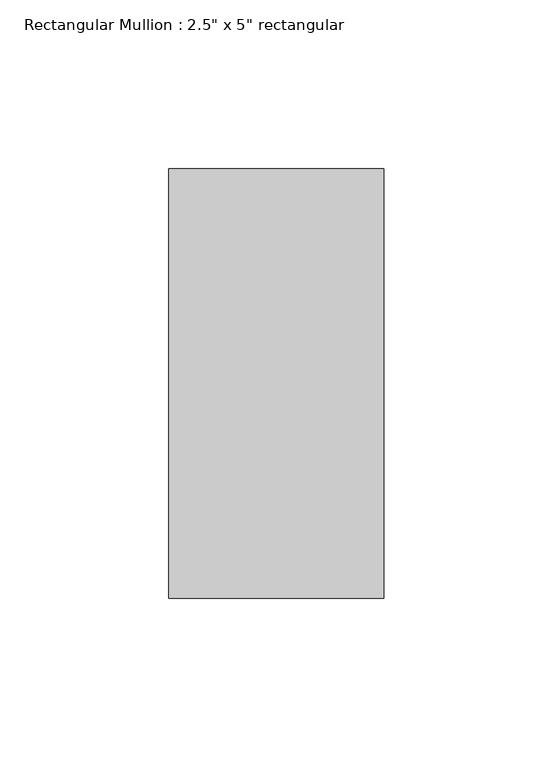
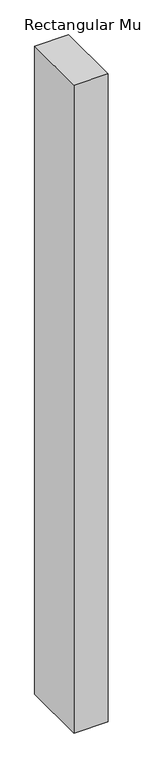
"""IFC4 building model written with IfcOpenShell, lengths in millimetres: member geometry."""

from ifc_helpers import new_model, si_unit, frame, origin, place, context, project, spatial, polyline, outline, extrude, source, transform, mapped, element, save


def member_ace9393b(model_context):
    return source(origin(), model_context, "Body", "SweptSolid", [
        extrude(outline(polyline([(0.0, 63.5), (0.0, -63.5), (-63.5, -63.5), (-63.5, 63.5), (0.0, 63.5)])), frame((0.0, 0.0, -1276.3500001), z_axis=(0.0, 0.0, 1.0), x_axis=(1.0, 0.0, 0.0)), (0.0, 0.0, 1.0), 1276.3500001),
    ])


if __name__ == "__main__":
    model = new_model("IFC4")
    model_context = context("Model", 3, world=origin())
    ifc_project = project(units=[si_unit("LENGTHUNIT", "METRE", prefix="MILLI")], contexts=[model_context])
    site = spatial("IfcSite", under=ifc_project)
    building = spatial("IfcBuilding", under=site)
    placement = place(None, origin())
    member_shape = member_ace9393b(model_context)
    element("IfcMember", 1, ObjectType="Rectangular Mullion : 2.5\" x 5\" rectangular", at=placement, inside=building, context=model_context, shape_type="MappedRepresentation", body=[
        mapped(member_shape, transform((0.0, 0.0, 0.0), x_axis=(1.0, 0.0, 0.0), y_axis=(0.0, 1.0, 0.0), z_axis=(0.0, 0.0, 1.0))),
    ])
    save(model, "model.ifc")

# Revit data of these elements
# Type "Rectangular Mullion : 2.5\" x 5\" rectangular"
#   built-in parameter 1007304 = 0.416667 (stored number, unit not read)
#   built-in parameter 1007301 = 0.104167 (stored number, unit not read)
#   built-in parameter 1007300 = 0.104167 (stored number, unit not read)
# Element 1 (IfcMember, "Rectangular Mullion : 2.5\" x 5\" rectangular")
#   Materials on its faces: "Aluminum"
# Materials
#   "Aluminum": class "Metal", colour RGB 247 247 247, transparency 0, Description = "Aluminum 6061", Cost = 0
